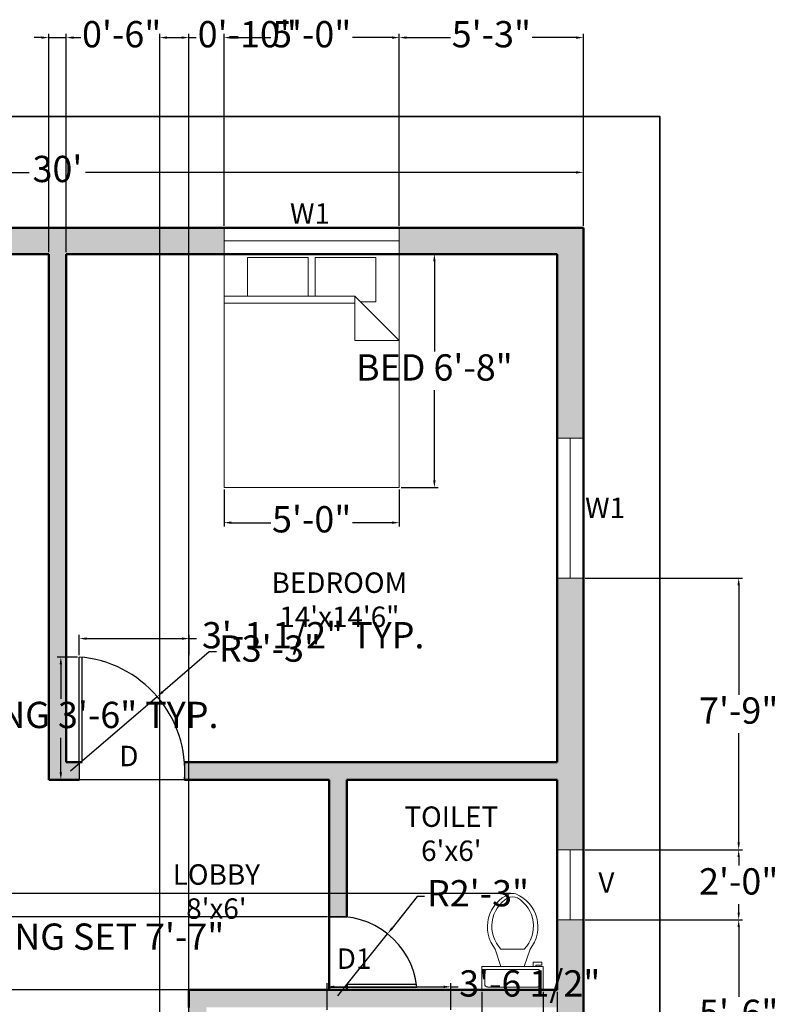
# Model space of a CAD drawing. Units: inches. Extents: x 6193 to 6719, y 6945 to 7563.
# Tile 4 of 4: x 6459 to 6719, y 7219 to 7556. Entities that reach past the tile are written whole.
import ezdxf

# ---------------------------------------------------------------- set-up
doc = ezdxf.new("R2010")
doc.units = ezdxf.units.IN
for name, color, linetype, lineweight in [('A-ANNO-DIMS', 2, 'Continuous', 18), ('A-ANNO-TEXT', 7, 'Continuous', 18), ('A-ANNO-TTLB', 7, 'Continuous', 35), ('A-AREA-IDEN', 7, 'Continuous', 25), ('A-DOOR', 3, 'Continuous', 25), ('A-FLOR-FIXT', 9, 'Continuous', 18), ('A-FURN', 8, 'Continuous', 18), ('A-GLAZ', 4, 'Continuous', 18), ('A-WALL', 7, 'Continuous', 50)]:
    doc.layers.add(name, color=color, linetype=linetype, lineweight=lineweight)
doc.layers.add('A-WALL-PATT', color=18, linetype='Continuous', lineweight=13, true_color=0x000000)
doc.styles.get("Standard").update_dxf_attribs({"font": 'arial.ttf'})
doc.dimstyles.new('ISO-25', dxfattribs={"dimtxt": 9, "dimasz": 2.5, "dimexe": 1.25, "dimexo": 0.625, "dimgap": 2, "dimtad": 0, "dimtih": 1, "dimtoh": 1, "dimdec": 1, "dimlunit": 4, "dimtxsty": 'Standard', "dimcen": 2.5, "dimadec": 0, "dimazin": 0, "dimtfac": 0.5, "dimtdec": 1, "dimtmove": 0, "dimatfit": 3, "dimfxl": 1, "dimarcsym": 0})

# ---------------------------------------------------------------- blocks, each defined once
blk = doc.blocks.new('Bed - Queen')
for p, q in [((0, -80.00003), (0, 0)), ((0, 0), (59.99999, 0)), ((59.99999, 0), (59.99999, -80.00003)), ((7.99999, -1.2), (28.79998, -1.2)), ((7.99999, -14.4), (7.99999, -1.2)), ((28.79998, -1.2), (28.79998, -14.4)), ((31.19999, -1.2), (51.99999, -1.2)), ((31.19999, -14.4), (31.19999, -1.2)), ((51.99999, -1.2), (51.99999, -16.4)), ((0, -14.4), (44.8, -14.4)), ((44.8, -16.8), (0, -16.8)), ((59.99999, -29.6), (44.8, -14.4)), ((44.8, -14.4), (44.8, -29.6)), ((51.99999, -16.4), (46.79936, -16.4)), ((44.8, -29.6), (59.99999, -29.6)), ((59.99999, -80.00003), (0, -80.00003))]:
    blk.add_line(p, q)
blk = doc.blocks.new('*U3')
for p, q in [((9.5, -6), (9.5, -2)), ((-10, -8.5), (-8, -8.5)), ((-10, -9.5), (-10, -8.5)), ((-7, -9.5), (-10, -9.5)), ((-8, -8.5), (-8, -8)), ((-7, -8), (-7, -9.5)), ((-4, -8), (-6, -14)), ((4, -8), (6, -14)), ((4, -14), (-4, -14))]:
    blk.add_line(p, q)
blk.add_lwpolyline([(10.5, -8), (10.5, 0), (-10.5, 0), (-10.5, -8)], close=True)
for points in [[(-9.5, -2), (-9.5, -6)], [(8.5, -1), (-8.5, -1)], [(-8.5, -7), (8.5, -7)]]:
    blk.add_lwpolyline(points)
for centre, radius, start, end in [((-8.62, -1.88), 0.884, 81.8699, 188.1301), ((8.62, -1.88), 0.884, 351.8699, 98.1301), ((-8.62, -6.12), 0.884, 171.8699, 278.1301), ((8.62, -6.12), 0.884, 261.8699, 8.1301), ((3.52, -21.58), 12.17, 141.4691, 247.9714), ((4.2, -21.82), 11.33, 136.3677, 238.9468), ((-3.52, -21.58), 12.17, 292.0284, 38.5307), ((-4.2, -21.82), 11.33, 301.053, 43.6321), ((0, -27.88), 4, 245.7318, 294.2682), ((0, -29), 4, 254.8605, 285.1395)]:
    blk.add_arc(centre, radius, start, end)
blk = doc.blocks.new('*D10')
at = {"layer": 'A-ANNO-DIMS', "color": 0, "lineweight": -2, "transparency": 16777216}
for p, q in [((6292.28, 7485.29), (6292.28, 7504.87)), ((6294.78, 7503.62), (6462.65, 7503.62)), ((6649.78, 7503.62), (6481.92, 7503.62)), ((6652.28, 7485.29), (6652.28, 7504.87))]:
    blk.add_line(p, q, dxfattribs=at)
at = {"layer": 'A-ANNO-DIMS', "color": 0, "transparency": 16777216}
for points in [[(6294.78, 7504.03), (6294.78, 7503.2), (6292.28, 7503.62)], [(6649.78, 7504.03), (6649.78, 7503.2), (6652.28, 7503.62)]]:
    blk.add_solid(points, dxfattribs=at)
at = {"layer": 'Defpoints', "color": 0, "transparency": 16777216}
for p in [(6652.28, 7503.62), (6292.28, 7484.66), (6652.28, 7484.66)]:
    blk.add_point(p, dxfattribs=at)
at = {"layer": 'A-ANNO-DIMS', "color": 0, "transparency": 16777216, "insert": (6472.28, 7503.62), "char_height": 9, "attachment_point": 5}
blk.add_mtext("30'", dxfattribs=at)
blk = doc.blocks.new('DOOR-SWING-36IN')
for p, q in [((0, 6), (0, 42)), ((1, 6), (1, 41.91)), ((0, 6), (0, 0)), ((36, 6), (36, 0))]:
    blk.add_line(p, q)
blk.add_arc((-3, 3), 39.12, 355.6013, 85.6013)
blk = doc.blocks.new('WIN-48IN')
for p, q in [((0, 48), (9, 48)), ((4.5, 48), (4.5, 0)), ((0, 0), (9, 0))]:
    blk.add_line(p, q)
blk = doc.blocks.new('*D16')
at = {"layer": 'A-ANNO-DIMS', "color": 0, "lineweight": -2, "transparency": 16777216}
for p, q in [((6589.91, 7475.66), (6602.53, 7475.66)), ((6601.28, 7473.16), (6601.28, 7442.26)), ((6601.28, 7398.16), (6601.28, 7429.07)), ((6589.91, 7395.66), (6602.53, 7395.66))]:
    blk.add_line(p, q, dxfattribs=at)
at = {"layer": 'A-ANNO-DIMS', "color": 0, "transparency": 16777216}
for points in [[(6600.87, 7473.16), (6601.7, 7473.16), (6601.28, 7475.66)], [(6600.87, 7398.16), (6601.7, 7398.16), (6601.28, 7395.66)]]:
    blk.add_solid(points, dxfattribs=at)
at = {"layer": 'Defpoints', "color": 0, "transparency": 16777216}
for p in [(6589.28, 7475.66), (6601.28, 7475.66), (6589.28, 7395.66)]:
    blk.add_point(p, dxfattribs=at)
at = {"layer": 'A-ANNO-DIMS', "color": 0, "transparency": 16777216, "insert": (6601.28, 7435.66), "char_height": 9, "attachment_point": 5}
blk.add_mtext('BED 6\'-8"', dxfattribs=at)
blk = doc.blocks.new('*D17')
at = {"layer": 'A-ANNO-DIMS', "color": 0, "lineweight": -2, "transparency": 16777216}
for p, q in [((6529.28, 7395.04), (6529.28, 7382.41)), ((6589.28, 7395.04), (6589.28, 7382.41)), ((6531.78, 7383.66), (6545.32, 7383.66)), ((6586.78, 7383.66), (6573.25, 7383.66))]:
    blk.add_line(p, q, dxfattribs=at)
at = {"layer": 'A-ANNO-DIMS', "color": 0, "transparency": 16777216}
for points in [[(6531.78, 7384.08), (6531.78, 7383.25), (6529.28, 7383.66)], [(6586.78, 7384.08), (6586.78, 7383.25), (6589.28, 7383.66)]]:
    blk.add_solid(points, dxfattribs=at)
at = {"layer": 'Defpoints', "color": 0, "transparency": 16777216}
for p in [(6529.28, 7395.66), (6589.28, 7395.66), (6589.28, 7383.66)]:
    blk.add_point(p, dxfattribs=at)
at = {"layer": 'A-ANNO-DIMS', "color": 0, "transparency": 16777216, "insert": (6559.28, 7383.66), "char_height": 9, "attachment_point": 5}
blk.add_mtext('5\'-0"', dxfattribs=at)
blk = doc.blocks.new('*D19')
at = {"layer": 'A-ANNO-DIMS', "color": 0, "lineweight": -2, "transparency": 16777216}
for p, q in [((6564.54, 7216.86), (6564.54, 7225.97)), ((6606.96, 7216.86), (6606.96, 7225.97)), ((6567.04, 7224.72), (6604.46, 7224.72)), ((6606.96, 7224.72), (6609.46, 7224.72))]:
    blk.add_line(p, q, dxfattribs=at)
at = {"layer": 'A-ANNO-DIMS', "color": 0, "transparency": 16777216}
for points in [[(6567.04, 7225.14), (6567.04, 7224.31), (6564.54, 7224.72)], [(6604.46, 7225.14), (6604.46, 7224.31), (6606.96, 7224.72)]]:
    blk.add_solid(points, dxfattribs=at)
at = {"layer": 'Defpoints', "color": 0, "transparency": 16777216}
for p in [(6606.96, 7224.72), (6564.54, 7216.24), (6606.96, 7216.24)]:
    blk.add_point(p, dxfattribs=at)
at = {"layer": 'A-ANNO-DIMS', "color": 0, "transparency": 16777216, "insert": (6633.91, 7224.72), "char_height": 9, "attachment_point": 5}
blk.add_mtext('3\'-6 1/2"', dxfattribs=at)
blk = doc.blocks.new('*D20')
at = {"layer": 'A-ANNO-DIMS', "color": 0, "lineweight": -2, "transparency": 16777216}
for p, q in [((6479.1, 7337.66), (6472.18, 7337.66)), ((6473.43, 7335.16), (6473.43, 7323.32)), ((6473.43, 7298.16), (6473.43, 7310.01)), ((6479.1, 7295.66), (6472.18, 7295.66))]:
    blk.add_line(p, q, dxfattribs=at)
at = {"layer": 'A-ANNO-DIMS', "color": 0, "transparency": 16777216}
for points in [[(6473.01, 7335.16), (6473.84, 7335.16), (6473.43, 7337.66)], [(6473.01, 7298.16), (6473.84, 7298.16), (6473.43, 7295.66)]]:
    blk.add_solid(points, dxfattribs=at)
at = {"layer": 'Defpoints', "color": 0, "transparency": 16777216}
for p in [(6473.43, 7337.66), (6479.73, 7337.66), (6479.73, 7295.66)]:
    blk.add_point(p, dxfattribs=at)
at = {"layer": 'A-ANNO-DIMS', "color": 0, "transparency": 16777216, "insert": (6473.43, 7316.66), "char_height": 9, "attachment_point": 5}
blk.add_mtext('D SWING 3\'-6" TYP.', dxfattribs=at)
blk = doc.blocks.new('*D21')
at = {"layer": 'A-ANNO-DIMS', "color": 0, "lineweight": -2, "transparency": 16777216}
for p, q in [((6479.73, 7338.29), (6479.73, 7345.21)), ((6482.23, 7343.96), (6514.88, 7343.96)), ((6517.38, 7338.29), (6517.38, 7345.21)), ((6517.38, 7343.96), (6519.88, 7343.96))]:
    blk.add_line(p, q, dxfattribs=at)
at = {"layer": 'A-ANNO-DIMS', "color": 0, "transparency": 16777216}
for points in [[(6482.23, 7344.38), (6482.23, 7343.55), (6479.73, 7343.96)], [(6514.88, 7344.38), (6514.88, 7343.55), (6517.38, 7343.96)]]:
    blk.add_solid(points, dxfattribs=at)
at = {"layer": 'Defpoints', "color": 0, "transparency": 16777216}
for p in [(6517.38, 7343.96), (6479.73, 7337.66), (6517.38, 7337.66)]:
    blk.add_point(p, dxfattribs=at)
at = {"layer": 'A-ANNO-DIMS', "color": 0, "transparency": 16777216, "insert": (6559.8, 7343.96), "char_height": 9, "attachment_point": 5}
blk.add_mtext('3\'-1 1/2" TYP.', dxfattribs=at)
blk = doc.blocks.new('*D22')
at = {"layer": 'A-ANNO-DIMS', "color": 0, "lineweight": -2, "transparency": 16777216}
for p, q in [((6336.22, 7253.77), (6336.22, 7239.49)), ((6427.22, 7253.77), (6427.22, 7239.49)), ((6338.72, 7240.74), (6424.72, 7240.74)), ((6427.22, 7240.74), (6429.72, 7240.74))]:
    blk.add_line(p, q, dxfattribs=at)
at = {"layer": 'A-ANNO-DIMS', "color": 0, "transparency": 16777216}
for points in [[(6338.72, 7241.16), (6338.72, 7240.33), (6336.22, 7240.74)], [(6424.72, 7241.16), (6424.72, 7240.33), (6427.22, 7240.74)]]:
    blk.add_solid(points, dxfattribs=at)
at = {"layer": 'Defpoints', "color": 0, "transparency": 16777216}
for p in [(6336.22, 7254.39), (6427.22, 7254.39), (6427.22, 7240.74)]:
    blk.add_point(p, dxfattribs=at)
at = {"layer": 'A-ANNO-DIMS', "color": 0, "transparency": 16777216, "insert": (6481.18, 7240.74), "char_height": 9, "attachment_point": 5}
blk.add_mtext('DINING SET 7\'-7"', dxfattribs=at)
blk = doc.blocks.new('*D39')
at = {"layer": 'A-ANNO-DIMS', "color": 0, "lineweight": -2, "transparency": 16777216}
for p, q in [((6652.91, 7247.66), (6706.68, 7247.66)), ((6705.43, 7245.16), (6705.43, 7221.26)), ((6705.43, 7184.16), (6705.43, 7208.07)), ((6652.91, 7181.66), (6706.68, 7181.66))]:
    blk.add_line(p, q, dxfattribs=at)
at = {"layer": 'A-ANNO-DIMS', "color": 0, "transparency": 16777216}
for points in [[(6705.01, 7245.16), (6705.84, 7245.16), (6705.43, 7247.66)], [(6705.01, 7184.16), (6705.84, 7184.16), (6705.43, 7181.66)]]:
    blk.add_solid(points, dxfattribs=at)
at = {"layer": 'Defpoints', "color": 0, "transparency": 16777216}
for p in [(6652.28, 7247.66), (6705.43, 7247.66), (6652.28, 7181.66)]:
    blk.add_point(p, dxfattribs=at)
at = {"layer": 'A-ANNO-DIMS', "color": 0, "transparency": 16777216, "insert": (6705.43, 7214.66), "char_height": 9, "attachment_point": 5}
blk.add_mtext('5\'-6"', dxfattribs=at)
blk = doc.blocks.new('*D40')
at = {"layer": 'A-ANNO-DIMS', "color": 0, "lineweight": -2, "transparency": 16777216}
for p, q in [((6652.91, 7271.66), (6706.68, 7271.66)), ((6705.43, 7269.16), (6705.43, 7266.26)), ((6705.43, 7250.16), (6705.43, 7253.07)), ((6652.91, 7247.66), (6706.68, 7247.66))]:
    blk.add_line(p, q, dxfattribs=at)
at = {"layer": 'A-ANNO-DIMS', "color": 0, "transparency": 16777216}
for points in [[(6705.01, 7269.16), (6705.84, 7269.16), (6705.43, 7271.66)], [(6705.01, 7250.16), (6705.84, 7250.16), (6705.43, 7247.66)]]:
    blk.add_solid(points, dxfattribs=at)
at = {"layer": 'Defpoints', "color": 0, "transparency": 16777216}
for p in [(6652.28, 7271.66), (6705.43, 7271.66), (6652.28, 7247.66)]:
    blk.add_point(p, dxfattribs=at)
at = {"layer": 'A-ANNO-DIMS', "color": 0, "transparency": 16777216, "insert": (6705.43, 7259.66), "char_height": 9, "attachment_point": 5}
blk.add_mtext('2\'-0"', dxfattribs=at)
blk = doc.blocks.new('*D41')
at = {"layer": 'A-ANNO-DIMS', "color": 0, "lineweight": -2, "transparency": 16777216}
for p, q in [((6652.91, 7364.66), (6706.68, 7364.66)), ((6705.43, 7362.16), (6705.43, 7324.76)), ((6705.43, 7274.16), (6705.43, 7311.57)), ((6652.91, 7271.66), (6706.68, 7271.66))]:
    blk.add_line(p, q, dxfattribs=at)
at = {"layer": 'A-ANNO-DIMS', "color": 0, "transparency": 16777216}
for points in [[(6705.01, 7362.16), (6705.84, 7362.16), (6705.43, 7364.66)], [(6705.01, 7274.16), (6705.84, 7274.16), (6705.43, 7271.66)]]:
    blk.add_solid(points, dxfattribs=at)
at = {"layer": 'Defpoints', "color": 0, "transparency": 16777216}
for p in [(6652.28, 7364.66), (6705.43, 7364.66), (6652.28, 7271.66)]:
    blk.add_point(p, dxfattribs=at)
at = {"layer": 'A-ANNO-DIMS', "color": 0, "transparency": 16777216, "insert": (6705.43, 7318.16), "char_height": 9, "attachment_point": 5}
blk.add_mtext('7\'-9"', dxfattribs=at)
blk = doc.blocks.new('*D42')
at = {"layer": 'A-ANNO-DIMS', "color": 0, "lineweight": -2, "transparency": 16777216}
for p, q in [((6589.28, 7485.29), (6589.28, 7551.02)), ((6591.78, 7549.77), (6606.82, 7549.77)), ((6649.78, 7549.77), (6634.75, 7549.77)), ((6652.28, 7485.29), (6652.28, 7551.02))]:
    blk.add_line(p, q, dxfattribs=at)
at = {"layer": 'A-ANNO-DIMS', "color": 0, "transparency": 16777216}
for points in [[(6591.78, 7550.19), (6591.78, 7549.36), (6589.28, 7549.77)], [(6649.78, 7550.19), (6649.78, 7549.36), (6652.28, 7549.77)]]:
    blk.add_solid(points, dxfattribs=at)
at = {"layer": 'Defpoints', "color": 0, "transparency": 16777216}
for p in [(6652.28, 7549.77), (6589.28, 7484.66), (6652.28, 7484.66)]:
    blk.add_point(p, dxfattribs=at)
at = {"layer": 'A-ANNO-DIMS', "color": 0, "transparency": 16777216, "insert": (6620.78, 7549.77), "char_height": 9, "attachment_point": 5}
blk.add_mtext('5\'-3"', dxfattribs=at)
blk = doc.blocks.new('*D43')
at = {"layer": 'A-ANNO-DIMS', "color": 0, "lineweight": -2, "transparency": 16777216}
for p, q in [((6529.28, 7485.29), (6529.28, 7551.02)), ((6531.78, 7549.77), (6545.32, 7549.77)), ((6586.78, 7549.77), (6573.25, 7549.77)), ((6589.28, 7485.29), (6589.28, 7551.02))]:
    blk.add_line(p, q, dxfattribs=at)
at = {"layer": 'A-ANNO-DIMS', "color": 0, "transparency": 16777216}
for points in [[(6531.78, 7550.19), (6531.78, 7549.36), (6529.28, 7549.77)], [(6586.78, 7550.19), (6586.78, 7549.36), (6589.28, 7549.77)]]:
    blk.add_solid(points, dxfattribs=at)
at = {"layer": 'Defpoints', "color": 0, "transparency": 16777216}
for p in [(6589.28, 7549.77), (6529.28, 7484.66), (6589.28, 7484.66)]:
    blk.add_point(p, dxfattribs=at)
at = {"layer": 'A-ANNO-DIMS', "color": 0, "transparency": 16777216, "insert": (6559.28, 7549.77), "char_height": 9, "attachment_point": 5}
blk.add_mtext('5\'-0"', dxfattribs=at)
blk = doc.blocks.new('*D51')
at = {"layer": 'A-ANNO-DIMS', "color": 0, "lineweight": -2, "transparency": 16777216}
for p, q in [((6507.28, 7092.29), (6507.28, 7551.02)), ((6509.78, 7549.77), (6514.78, 7549.77)), ((6517.28, 7092.29), (6517.28, 7551.02)), ((6517.28, 7549.77), (6519.78, 7549.77))]:
    blk.add_line(p, q, dxfattribs=at)
at = {"layer": 'A-ANNO-DIMS', "color": 0, "transparency": 16777216}
for points in [[(6509.78, 7550.19), (6509.78, 7549.36), (6507.28, 7549.77)], [(6514.78, 7550.19), (6514.78, 7549.36), (6517.28, 7549.77)]]:
    blk.add_solid(points, dxfattribs=at)
at = {"layer": 'Defpoints', "color": 0, "transparency": 16777216}
for p in [(6517.28, 7549.77), (6507.28, 7091.66), (6517.28, 7091.66)]:
    blk.add_point(p, dxfattribs=at)
at = {"layer": 'A-ANNO-DIMS', "color": 0, "transparency": 16777216, "insert": (6537.24, 7549.77), "char_height": 9, "attachment_point": 5}
blk.add_mtext('0\'-10"', dxfattribs=at)
blk = doc.blocks.new('*D53')
at = {"layer": 'A-ANNO-DIMS', "color": 0, "lineweight": -2, "transparency": 16777216}
for p, q in [((6564.66, 7248.66), (6215.49, 7248.66)), ((6216.74, 7246.16), (6216.74, 7242.68)), ((6216.74, 7226.16), (6216.74, 7229.64)), ((6564.66, 7223.66), (6215.49, 7223.66))]:
    blk.add_line(p, q, dxfattribs=at)
at = {"layer": 'A-ANNO-DIMS', "color": 0, "transparency": 16777216}
for points in [[(6216.32, 7246.16), (6217.16, 7246.16), (6216.74, 7248.66)], [(6216.32, 7226.16), (6217.16, 7226.16), (6216.74, 7223.66)]]:
    blk.add_solid(points, dxfattribs=at)
at = {"layer": 'Defpoints', "color": 0, "transparency": 16777216}
for p in [(6216.74, 7248.66), (6565.28, 7248.66), (6565.28, 7223.66)]:
    blk.add_point(p, dxfattribs=at)
at = {"layer": 'A-ANNO-DIMS', "color": 0, "transparency": 16777216, "insert": (6216.74, 7236.16), "char_height": 9, "attachment_point": 5}
blk.add_mtext('2\'-1"', dxfattribs=at)
blk = doc.blocks.new('*D54')
at = {"layer": 'A-ANNO-DIMS', "color": 0, "lineweight": -2, "transparency": 16777216}
for p, q in [((6617.56, 7223.04), (6617.56, 6957.2)), ((6638.56, 7223.04), (6638.56, 6957.2)), ((6620.06, 6958.45), (6636.06, 6958.45)), ((6638.56, 6958.45), (6641.06, 6958.45))]:
    blk.add_line(p, q, dxfattribs=at)
at = {"layer": 'A-ANNO-DIMS', "color": 0, "transparency": 16777216}
for points in [[(6620.06, 6958.86), (6620.06, 6958.03), (6617.56, 6958.45)], [(6636.06, 6958.86), (6636.06, 6958.03), (6638.56, 6958.45)]]:
    blk.add_solid(points, dxfattribs=at)
at = {"layer": 'Defpoints', "color": 0, "transparency": 16777216}
for p in [(6617.56, 7223.66), (6638.56, 7223.66), (6638.56, 6958.45)]:
    blk.add_point(p, dxfattribs=at)
at = {"layer": 'A-ANNO-DIMS', "color": 0, "transparency": 16777216, "insert": (6654.6, 6958.45), "char_height": 9, "attachment_point": 5}
blk.add_mtext('1\'-9"', dxfattribs=at)
blk = doc.blocks.new('*D55')
at = {"layer": 'A-ANNO-DIMS', "color": 0, "lineweight": -2, "transparency": 16777216}
for p, q in [((6627.43, 7256.66), (6215.49, 7256.66)), ((6216.74, 7254.16), (6216.74, 7246.76)), ((6216.74, 7226.16), (6216.74, 7233.57)), ((6616.93, 7223.66), (6215.49, 7223.66))]:
    blk.add_line(p, q, dxfattribs=at)
at = {"layer": 'A-ANNO-DIMS', "color": 0, "transparency": 16777216}
for points in [[(6216.32, 7254.16), (6217.16, 7254.16), (6216.74, 7256.66)], [(6216.32, 7226.16), (6217.16, 7226.16), (6216.74, 7223.66)]]:
    blk.add_solid(points, dxfattribs=at)
at = {"layer": 'Defpoints', "color": 0, "transparency": 16777216}
for p in [(6216.74, 7256.66), (6628.06, 7256.66), (6617.56, 7223.66)]:
    blk.add_point(p, dxfattribs=at)
at = {"layer": 'A-ANNO-DIMS', "color": 0, "transparency": 16777216, "insert": (6216.74, 7240.16), "char_height": 9, "attachment_point": 5}
blk.add_mtext('2\'-9"', dxfattribs=at)
blk = doc.blocks.new('*D56')
at = {"layer": 'A-ANNO-DIMS', "color": 0, "lineweight": -2, "transparency": 16777216}
for p, q in [((6638.56, 7223.04), (6638.56, 6957.2)), ((6643.28, 7223.04), (6643.28, 6957.2)), ((6636.06, 6958.45), (6633.56, 6958.45)), ((6638.56, 6958.45), (6643.28, 6958.45)), ((6645.78, 6958.45), (6648.28, 6958.45))]:
    blk.add_line(p, q, dxfattribs=at)
at = {"layer": 'A-ANNO-DIMS', "color": 0, "transparency": 16777216}
for points in [[(6636.06, 6958.86), (6636.06, 6958.03), (6638.56, 6958.45)], [(6645.78, 6958.86), (6645.78, 6958.03), (6643.28, 6958.45)]]:
    blk.add_solid(points, dxfattribs=at)
at = {"layer": 'Defpoints', "color": 0, "transparency": 16777216}
for p in [(6638.56, 7223.66), (6643.28, 7223.66), (6643.28, 6958.45)]:
    blk.add_point(p, dxfattribs=at)
at = {"layer": 'A-ANNO-DIMS', "color": 0, "transparency": 16777216, "insert": (6672.73, 6958.45), "char_height": 9, "attachment_point": 5}
blk.add_mtext('0\'-4 1/2"', dxfattribs=at)
blk = doc.blocks.new('*D64')
at = {"layer": 'A-ANNO-DIMS', "color": 0, "lineweight": -2, "transparency": 16777216}
for p, q in [((6466.78, 7549.77), (6464.28, 7549.77)), ((6469.28, 7476.29), (6469.28, 7551.02)), ((6469.28, 7549.77), (6475.28, 7549.77)), ((6475.28, 7476.29), (6475.28, 7551.02)), ((6477.78, 7549.77), (6480.28, 7549.77))]:
    blk.add_line(p, q, dxfattribs=at)
at = {"layer": 'A-ANNO-DIMS', "color": 0, "transparency": 16777216}
for points in [[(6466.78, 7550.19), (6466.78, 7549.36), (6469.28, 7549.77)], [(6477.78, 7550.19), (6477.78, 7549.36), (6475.28, 7549.77)]]:
    blk.add_solid(points, dxfattribs=at)
at = {"layer": 'Defpoints', "color": 0, "transparency": 16777216}
for p in [(6475.28, 7549.77), (6469.28, 7475.66), (6475.28, 7475.66)]:
    blk.add_point(p, dxfattribs=at)
at = {"layer": 'A-ANNO-DIMS', "color": 0, "transparency": 16777216, "insert": (6494.25, 7549.77), "char_height": 9, "attachment_point": 5}
blk.add_mtext('0\'-6"', dxfattribs=at)
blk = doc.blocks.new('*D66')
at = {"layer": 'A-ANNO-DIMS', "color": 0, "lineweight": -2, "transparency": 16777216}
for p, q in [((6524.24, 7339.39), (6508.32, 7325.75)), ((6526.74, 7339.39), (6524.24, 7339.39)), ((6476.73, 7298.66), (6506.43, 7324.12))]:
    blk.add_line(p, q, dxfattribs=at)
at = {"layer": 'A-ANNO-DIMS', "color": 0, "transparency": 16777216}
blk.add_solid([(6508.05, 7326.06), (6508.59, 7325.43), (6506.43, 7324.12)], dxfattribs=at)
at = {"layer": 'Defpoints', "color": 0, "transparency": 16777216}
for p in [(6506.43, 7324.12), (6476.73, 7298.66)]:
    blk.add_point(p, dxfattribs=at)
at = {"layer": 'A-ANNO-DIMS', "color": 0, "transparency": 16777216, "insert": (6545.01, 7339.39), "char_height": 9, "attachment_point": 5}
blk.add_mtext('R3\'-3"', dxfattribs=at)
blk = doc.blocks.new('*D67')
at = {"layer": 'A-ANNO-DIMS', "color": 0, "lineweight": -2, "transparency": 16777216}
for p, q in [((6595.44, 7255.6), (6586.82, 7244.83)), ((6597.94, 7255.6), (6595.44, 7255.6)), ((6568.28, 7221.66), (6585.26, 7242.88))]:
    blk.add_line(p, q, dxfattribs=at)
at = {"layer": 'A-ANNO-DIMS', "color": 0, "transparency": 16777216}
blk.add_solid([(6586.49, 7245.09), (6587.14, 7244.57), (6585.26, 7242.88)], dxfattribs=at)
at = {"layer": 'Defpoints', "color": 0, "transparency": 16777216}
for p in [(6585.26, 7242.88), (6568.28, 7221.66)]:
    blk.add_point(p, dxfattribs=at)
at = {"layer": 'A-ANNO-DIMS', "color": 0, "transparency": 16777216, "insert": (6616.21, 7255.6), "char_height": 9, "attachment_point": 5}
blk.add_mtext('R2\'-3"', dxfattribs=at)

msp = doc.modelspace()

# ---------------------------------------------------------------- hatches: boundary and pattern name
at = {"layer": 'A-WALL-PATT'}
h = msp.add_hatch(color=256, dxfattribs=at)
h.dxf.hatch_style = 1
h.paths.add_polyline_path([(6529.28, 7484.66), (6292.28, 7484.66), (6292.28, 7436.66), (6301.28, 7436.66), (6301.28, 7475.66), (6469.28, 7475.66), (6469.28, 7295.66), (6475.28, 7295.66), (6479.73, 7295.66), (6479.73, 7301.66), (6475.28, 7301.66), (6475.28, 7475.66), (6529.28, 7475.66)])
h.paths.add_polyline_path([(6652.28, 7484.66), (6589.28, 7484.66), (6589.28, 7475.66), (6643.28, 7475.66), (6643.28, 7412.66), (6652.28, 7412.66)])
h.paths.add_polyline_path([(6652.28, 7364.66), (6643.28, 7364.66), (6643.28, 7301.66), (6515.73, 7301.66, -0.038405), (6515.73, 7295.66), (6565.28, 7295.66), (6565.28, 7248.66, -0.055385), (6571.28, 7248.66), (6571.28, 7295.66), (6643.28, 7295.66), (6643.28, 7271.66), (6652.28, 7271.66)])
h.paths.add_polyline_path([(6652.28, 7247.66), (6643.28, 7247.66), (6643.28, 7223.66), (6571.28, 7223.66), (6565.28, 7223.66), (6517.28, 7223.66), (6517.28, 7217.66), (6517.28, 7135.82, -0.038405), (6523.28, 7135.82), (6523.28, 7217.66), (6565.28, 7217.66), (6571.28, 7217.66), (6643.28, 7217.66), (6643.28, 7181.66), (6652.28, 7181.66)])
h.paths.add_polyline_path([(6301.28, 7217.66), (6410.54, 7217.66), (6410.54, 7223.66), (6301.28, 7223.66), (6301.28, 7259.66), (6292.28, 7259.66), (6292.28, 7139.66), (6301.28, 7139.66)])
h.paths.add_polyline_path([(6301.28, 7343.66), (6361.63, 7343.66), (6361.63, 7349.66), (6301.28, 7349.66), (6301.28, 7388.66), (6292.28, 7388.66), (6292.28, 7307.66), (6301.28, 7307.66)], flags=17)
h.paths.add_polyline_path([(6301.28, 7091.66), (6292.28, 7091.66), (6292.28, 7004.66), (6302.28, 7004.66), (6302.28, 7013.66), (6301.28, 7013.66)])
h.paths.add_polyline_path([(6395.41, 7013.66), (6338.28, 7013.66, -0.055385), (6338.28, 7004.66), (6395.41, 7004.66)])
h.paths.add_polyline_path([(6652.28, 7028.66), (6643.28, 7028.66), (6643.28, 7013.66), (6443.41, 7013.66), (6443.41, 7004.66), (6652.28, 7004.66)])
h.paths.add_polyline_path([(6652.28, 7133.66), (6643.28, 7133.66), (6643.28, 7097.66), (6523.28, 7097.66), (6517.28, 7097.66), (6517.28, 7091.66), (6523.28, 7091.66), (6643.28, 7091.66), (6643.28, 7076.66), (6652.28, 7076.66)])
h.paths.add_polyline_path([(6517.28, 7097.66), (6507.28, 7097.66), (6507.28, 7091.66), (6517.28, 7091.66)])

# ---------------------------------------------------------------- linework, layer by layer
at = {"layer": 'A-ANNO-TTLB'}
msp.add_lwpolyline([(6243.74, 7522.77), (6678.43, 7522.77), (6678.43, 6985.45), (6243.74, 6985.45)], close=True, dxfattribs=at)
at = {"layer": 'A-DOOR'}
for p, q in [((6515.73, 7295.66), (6479.73, 7295.66)), ((6565.28, 7248.66), (6571.28, 7248.66)), ((6571.28, 7225.66), (6595.15, 7225.66)), ((6565.28, 7224.66), (6571.28, 7224.66)), ((6571.28, 7224.66), (6595.28, 7224.66))]:
    msp.add_line(p, q, dxfattribs=at)
msp.add_arc((6568.28, 7221.66), 27.17, 6.3402, 96.3402, dxfattribs=at)
at = {"layer": 'A-GLAZ'}
for p, q in [((6529.28, 7475.66), (6529.28, 7484.66)), ((6589.28, 7475.66), (6589.28, 7484.66)), ((6529.28, 7480.16), (6589.28, 7480.16)), ((6643.28, 7271.66), (6652.28, 7271.66)), ((6647.78, 7271.66), (6647.78, 7247.66)), ((6643.28, 7247.66), (6652.28, 7247.66))]:
    msp.add_line(p, q, dxfattribs=at)
at = {"layer": 'A-WALL'}
for p, q in [((6292.28, 7484.66), (6652.28, 7484.66)), ((6652.28, 7484.66), (6652.28, 7004.66)), ((6301.28, 7475.66), (6469.28, 7475.66)), ((6469.28, 7295.66), (6469.28, 7475.66)), ((6475.28, 7475.66), (6643.28, 7475.66)), ((6475.28, 7301.66), (6475.28, 7475.66)), ((6643.28, 7475.66), (6643.28, 7301.66)), ((6469.28, 7295.66), (6469.28, 7343.66)), ((6475.28, 7301.66), (6480.73, 7301.66)), ((6515.73, 7301.66), (6643.28, 7301.66)), ((6475.28, 7295.66), (6469.28, 7295.66)), ((6475.28, 7295.66), (6479.73, 7295.66)), ((6515.73, 7295.66), (6565.28, 7295.66)), ((6565.28, 7295.66), (6565.28, 7223.66)), ((6571.28, 7295.66), (6571.28, 7248.66)), ((6571.28, 7295.66), (6643.28, 7295.66)), ((6643.28, 7295.66), (6643.28, 7223.66)), ((6571.28, 7225.66), (6571.28, 7223.66)), ((6565.28, 7223.66), (6517.28, 7223.66)), ((6517.28, 7217.66), (6517.28, 7223.66)), ((6565.28, 7223.66), (6571.28, 7223.66)), ((6571.28, 7223.66), (6643.28, 7223.66))]:
    msp.add_line(p, q, dxfattribs=at)

# ---------------------------------------------------------------- block references
at = {"layer": 'A-DOOR'}
msp.add_blockref('DOOR-SWING-36IN', (6479.73, 7295.66), dxfattribs=at)
at = {"layer": 'A-FLOR-FIXT', "rotation": 180}
msp.add_blockref('*U3', (6628.06, 7223.66), dxfattribs=at)
at = {"layer": 'A-FURN'}
msp.add_blockref('Bed - Queen', (6529.28, 7475.66), dxfattribs=at)
at = {"layer": 'A-GLAZ'}
msp.add_blockref('WIN-48IN', (6643.28, 7364.66), dxfattribs=at)

# ---------------------------------------------------------------- texts
at = {"layer": 'A-ANNO-TEXT', "char_height": 7, "attachment_point": 1}
for s, width, insert in [('\\pxqc;W1', 21.3946, (6548.01, 7493.02)), ('\\pxqc;W1', 21.3946, (6649.01, 7392.25)), ('\\pxqc;D', 20.1481, (6486.66, 7307.26)), ('\\pxqc;V', 21.3946, (6649.45, 7263.93)), ('\\pxqc;D1', 20.1481, (6563.71, 7237.87))]:
    msp.add_mtext_dynamic_manual_height_columns(s, width=width, gutter_width=12.5, heights=[0], dxfattribs=dict(at, insert=insert))
at = {"layer": 'A-AREA-IDEN', "char_height": 7, "attachment_point": 1}
for s, width, insert in [('\\pxqc;{\\fArial|b1|i0|c0|p34;BEDROOM\\P14\'x14\'6"}', 125.0606, (6506.23, 7366.62)), ("\\pxqc;{\\fArial|b1|i0|c0|p34;TOILET\\P6'x6'}", 61.4012, (6576.37, 7286.49)), ("\\pxqc;{\\fArial|b1|i0|c0|p34;LOBBY\\P8'x6'}", 52.0396, (6500.65, 7266.68))]:
    msp.add_mtext_dynamic_manual_height_columns(s, width=width, gutter_width=12.5, heights=[0], dxfattribs=dict(at, insert=insert))

# ---------------------------------------------------------------- dimensions: what is measured, and where the dimension line sits
at = {"layer": 'A-ANNO-DIMS'}
for base, p1, p2, override, picture, middle in [((6475.28, 7549.77), (6469.28, 7475.66), (6475.28, 7475.66), {"dimdec": 1, "dimlfac": 1, "dimrnd": 0, "dimzin": 1, "dimdsep": 46, "dimlunit": 4, "dimfrac": 2}, '*D64', (6494.25, 7549.77)), ((6517.28, 7549.77), (6507.28, 7091.66), (6517.28, 7091.66), {"dimdec": 1, "dimlfac": 1, "dimrnd": 0, "dimzin": 1, "dimdsep": 46, "dimlunit": 4, "dimfrac": 2}, '*D51', (6537.24, 7549.77)), ((6589.28, 7549.77), (6529.28, 7484.66), (6589.28, 7484.66), {"dimdec": 1, "dimlfac": 1, "dimrnd": 0, "dimzin": 1, "dimdsep": 46, "dimlunit": 4, "dimfrac": 2}, '*D43', (6559.28, 7549.77)), ((6652.28, 7549.77), (6589.28, 7484.66), (6652.28, 7484.66), {"dimdec": 1, "dimlfac": 1, "dimrnd": 0, "dimzin": 1, "dimdsep": 46, "dimlunit": 4, "dimfrac": 2}, '*D42', (6620.78, 7549.77)), ((6652.28, 7503.62), (6292.28, 7484.66), (6652.28, 7484.66), {"dimclrd": 0, "dimclre": 0, "dimclrt": 0}, '*D10', (6472.28, 7503.62)), ((6589.28, 7383.66), (6529.28, 7395.66), (6589.28, 7395.66), {"dimdec": 1, "dimlfac": 1, "dimrnd": 0, "dimzin": 1, "dimdsep": 46, "dimlunit": 4, "dimfrac": 2}, '*D17', (6559.28, 7383.66)), ((6606.96, 7224.72), (6564.54, 7216.24), (6606.96, 7216.24), {"dimdec": 1, "dimlfac": 1, "dimrnd": 0, "dimzin": 1, "dimdsep": 46, "dimlunit": 4, "dimfrac": 2}, '*D19', (6633.91, 7224.72)), ((6638.56, 6958.45), (6617.56, 7223.66), (6638.56, 7223.66), {"dimdec": 1, "dimlfac": 1, "dimrnd": 0, "dimzin": 1, "dimdsep": 46, "dimlunit": 4, "dimfrac": 2}, '*D54', (6654.6, 6958.45)), ((6643.28, 6958.45), (6638.56, 7223.66), (6643.28, 7223.66), {"dimdec": 1, "dimlfac": 1, "dimrnd": 0, "dimzin": 1, "dimdsep": 46, "dimlunit": 4, "dimfrac": 2}, '*D56', (6672.73, 6958.45))]:
    dim = msp.add_linear_dim(base=base, p1=p1, p2=p2, dimstyle='ISO-25', override=override, dxfattribs=at)
    dim.commit()
    dim.dimension.update_dxf_attribs({"geometry": picture, "text_midpoint": middle})
for base, p1, p2, text, picture, middle in [((6601.28, 7475.66), (6589.28, 7395.66), (6589.28, 7475.66), 'BED <>', '*D16', (6601.28, 7435.66)), ((6473.43, 7337.66), (6479.73, 7295.66), (6479.73, 7337.66), 'D SWING <> TYP.', '*D20', (6473.43, 7316.66))]:
    dim = msp.add_linear_dim(base=base, p1=p1, p2=p2, angle=90, text=text, dimstyle='ISO-25', override={"dimdec": 1, "dimlfac": 1, "dimrnd": 0, "dimzin": 1, "dimdsep": 46, "dimlunit": 4, "dimfrac": 2}, dxfattribs=at)
    dim.commit()
    dim.dimension.update_dxf_attribs({"geometry": picture, "text_midpoint": middle})
for base, p1, p2, text, picture, middle in [((6517.3838, 7343.9631), (6479.7269, 7337.6631), (6517.3838, 7337.6631), '<> TYP.', '*D21', (6559.7961, 7343.9631)), ((6427.22, 7240.74), (6336.22, 7254.39), (6427.22, 7254.39), 'DINING SET <>', '*D22', (6481.18, 7240.74))]:
    dim = msp.add_linear_dim(base=base, p1=p1, p2=p2, text=text, dimstyle='ISO-25', override={"dimdec": 1, "dimlfac": 1, "dimrnd": 0, "dimzin": 1, "dimdsep": 46, "dimlunit": 4, "dimfrac": 2}, dxfattribs=at)
    dim.commit()
    dim.dimension.update_dxf_attribs({"geometry": picture, "text_midpoint": middle})
for base, p1, p2, picture, middle in [((6705.43, 7364.66), (6652.28, 7271.66), (6652.28, 7364.66), '*D41', (6705.43, 7318.16)), ((6705.43, 7271.66), (6652.28, 7247.66), (6652.28, 7271.66), '*D40', (6705.43, 7259.66)), ((6216.74, 7256.66), (6617.56, 7223.66), (6628.06, 7256.66), '*D55', (6216.74, 7240.16)), ((6216.74, 7248.66), (6565.28, 7223.66), (6565.28, 7248.66), '*D53', (6216.74, 7236.16)), ((6705.43, 7247.66), (6652.28, 7181.66), (6652.28, 7247.66), '*D39', (6705.43, 7214.66))]:
    dim = msp.add_linear_dim(base=base, p1=p1, p2=p2, angle=90, dimstyle='ISO-25', override={"dimdec": 1, "dimlfac": 1, "dimrnd": 0, "dimzin": 1, "dimdsep": 46, "dimlunit": 4, "dimfrac": 2}, dxfattribs=at)
    dim.commit()
    dim.dimension.update_dxf_attribs({"geometry": picture, "text_midpoint": middle})
for center, mpoint, picture, middle in [((6476.73, 7298.66), (6506.43, 7324.12), '*D66', (6545.01, 7339.39)), ((6568.28, 7221.66), (6585.26, 7242.88), '*D67', (6616.21, 7255.6))]:
    dim = msp.add_radius_dim(center=center, mpoint=mpoint, dimstyle='ISO-25', override={"dimdec": 1, "dimlfac": 1, "dimrnd": 0, "dimzin": 1, "dimdsep": 46, "dimlunit": 4, "dimfrac": 2}, dxfattribs=at)
    dim.commit()
    dim.dimension.update_dxf_attribs({"geometry": picture, "text_midpoint": middle, "dimtype": 164})

doc.saveas('drawing.dxf')
